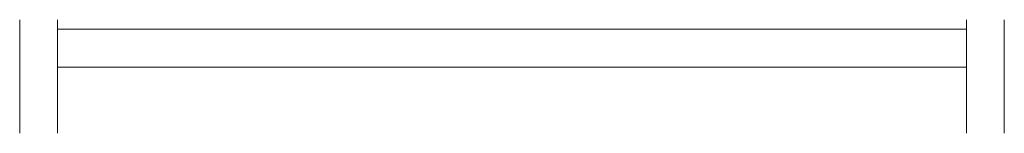
# Model space of a CAD drawing. Units: inches. Extents: x 25 to 82118, y 10 to 6494.
# Tile 9 of 9: x 82066 to 82118, y 6488 to 6494. Entities that reach past the tile are written whole.
import ezdxf

# ---------------------------------------------------------------- set-up
doc = ezdxf.new("R2010")
doc.units = ezdxf.units.IN
doc.header["$MEASUREMENT"] = 0
doc.layers.add('A-GLAZ', color=4, linetype='Continuous', lineweight=18)

msp = doc.modelspace()

# ---------------------------------------------------------------- linework, layer by layer
at = {"layer": 'A-GLAZ'}
for p, q in [((82065.504, 6487.638), (82065.504, 6493.638)), ((82067.504, 6487.638), (82067.504, 6493.638)), ((82115.504, 6487.638), (82115.504, 6493.638)), ((82117.504, 6487.638), (82117.504, 6493.638)), ((82067.504, 6493.138), (82115.504, 6493.138)), ((82067.504, 6491.138), (82115.504, 6491.138))]:
    msp.add_line(p, q, dxfattribs=at)

doc.saveas('drawing.dxf')
